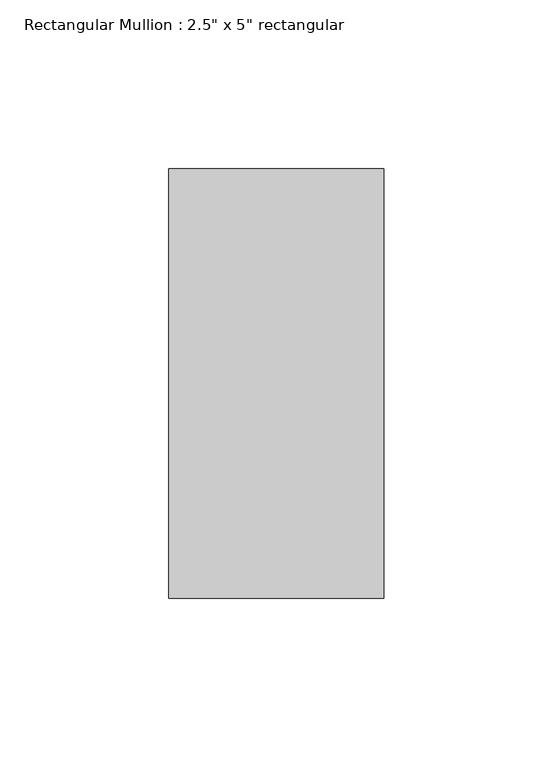
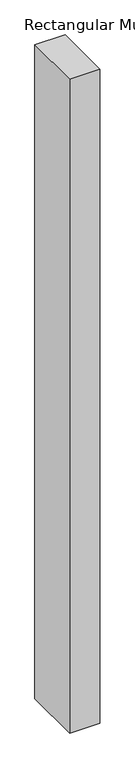
"""IFC4 building model written with IfcOpenShell, lengths in millimetres: member geometry."""

from ifc_helpers import new_model, si_unit, frame, origin, place, context, project, spatial, polyline, outline, extrude, source, transform, mapped, element, save


def member_39e99675(model_context):
    return source(origin(), model_context, "Body", "SweptSolid", [
        extrude(outline(polyline([(31.75, 63.5), (31.75, -63.5), (-31.75, -63.5), (-31.75, 63.5), (31.75, 63.5)])), frame((0.0, 0.0, -1457.1797686), z_axis=(0.0, 0.0, 1.0), x_axis=(1.0, 0.0, 0.0)), (0.0, 0.0, 1.0), 1457.1797686),
    ])


if __name__ == "__main__":
    model = new_model("IFC4")
    model_context = context("Model", 3, world=origin())
    ifc_project = project(units=[si_unit("LENGTHUNIT", "METRE", prefix="MILLI")], contexts=[model_context])
    site = spatial("IfcSite", under=ifc_project)
    building = spatial("IfcBuilding", under=site)
    placement = place(None, origin())
    member_shape = member_39e99675(model_context)
    element("IfcMember", 1, ObjectType="Rectangular Mullion : 2.5\" x 5\" rectangular", at=placement, inside=building, context=model_context, shape_type="MappedRepresentation", body=[
        mapped(member_shape, transform((0.0, 0.0, 0.0), x_axis=(1.0, 0.0, 0.0), y_axis=(0.0, 1.0, 0.0), z_axis=(0.0, 0.0, 1.0))),
    ])
    save(model, "model.ifc")

# Revit data of these elements
# Type "Rectangular Mullion : 2.5\" x 5\" rectangular"
#   built-in parameter 1007304 = 0.416667 (stored number, unit not read)
#   built-in parameter 1007301 = 0.104167 (stored number, unit not read)
#   built-in parameter 1007300 = 0.104167 (stored number, unit not read)
# Element 1 (IfcMember, "Rectangular Mullion : 2.5\" x 5\" rectangular")
#   Materials on its faces: "Aluminum"
# Materials
#   "Aluminum": class "Metal", colour RGB 247 247 247, transparency 0, Description = "Aluminum 6061", Cost = 0
